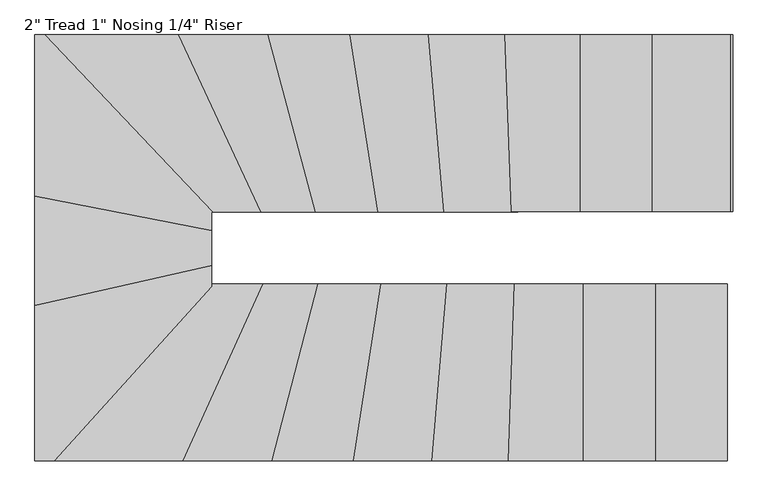
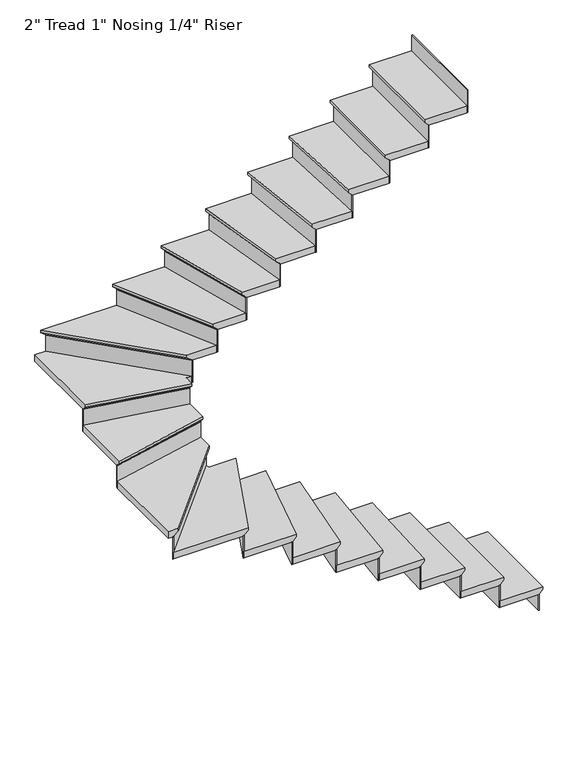
"""IFC4 building model written with IfcOpenShell, lengths in millimetres: stair flight geometry."""

from ifc_helpers import new_model, si_unit, origin, place, context, project, spatial, faceted_brep, source, transform, mapped, element, save


def stair_flight_7ceb0e75(model_context):
    return source(origin(), model_context, "Body", "Brep", [
        faceted_brep([(-10636.560337, -2913.3366944, 319.6166667), (-10636.560337, -2913.3366944, 338.6666667), (-10636.560337, -3599.1366944, 338.6666667), (-10636.560337, -3599.1366944, 319.6166667), (-10661.960337, -2913.3366944, 294.2166667), (-10661.960337, -3599.1366944, 294.2166667), (-10941.360337, -2913.3366944, 338.6666667), (-10941.360337, -3599.1366944, 338.6666667), (-10661.960337, -3599.1366944, 287.8666667), (-10941.360337, -3599.1366944, 287.8666667), (-10941.360337, -2913.3366944, 287.8666667), (-10661.960337, -2913.3366944, 287.8666667)], [[[0, 1, 2, 3]], [[4, 0, 3, 5]], [[2, 1, 6, 7]], [[8, 9, 10, 11]], [[2, 7, 9, 8, 5, 3]], [[8, 11, 4, 5]], [[6, 1, 0, 4, 11, 10]], [[7, 6, 10, 9]]]),
        faceted_brep([(-10661.960337, -2913.3366944, 287.8666667), (-10661.960337, -2913.3366944, 169.3333333), (-10668.310337, -2913.3366944, 169.3333333), (-10668.310337, -2913.3366944, 287.8666667), (-10661.960337, -3599.1366944, 287.8666667), (-10668.310337, -3599.1366944, 287.8666667), (-10668.310337, -3599.1366944, 169.3333333), (-10661.960337, -3599.1366944, 169.3333333)], [[[0, 1, 2, 3]], [[4, 5, 6, 7]], [[1, 0, 4, 7]], [[2, 1, 7, 6]], [[3, 2, 6, 5]], [[0, 3, 5, 4]]]),
        faceted_brep([(-10941.360337, -2913.3366944, 457.2), (-10941.360337, -2913.3366944, 287.8666667), (-10947.710337, -2913.3366944, 287.8666667), (-10947.710337, -2913.3366944, 457.2), (-10941.360337, -3599.1366944, 457.2), (-10947.710337, -3599.1366944, 457.2), (-10947.710337, -3599.1366944, 287.8666667), (-10941.360337, -3599.1366944, 287.8666667)], [[[0, 1, 2, 3]], [[4, 5, 6, 7]], [[1, 0, 4, 7]], [[2, 1, 7, 6]], [[3, 2, 6, 5]], [[0, 3, 5, 4]]]),
        faceted_brep([(-10915.960337, -3599.1366944, 508.0), (-10915.960337, -2913.3366944, 508.0), (-11220.760337, -2913.3366944, 508.0), (-11220.760337, -3599.1366944, 508.0), (-10941.360337, -3599.1366944, 457.2), (-11220.760337, -3599.1366944, 457.2), (-11220.760337, -2913.3366944, 457.2), (-10941.360337, -2913.3366944, 457.2), (-10941.360337, -3599.1366944, 463.55), (-10915.960337, -3599.1366944, 488.95), (-10941.360337, -2913.3366944, 463.55), (-10915.960337, -2913.3366944, 488.95)], [[[0, 1, 2, 3]], [[4, 5, 6, 7]], [[0, 3, 5, 4, 8, 9]], [[4, 7, 10, 8]], [[2, 1, 11, 10, 7, 6]], [[3, 2, 6, 5]], [[11, 1, 0, 9]], [[10, 11, 9, 8]]]),
        faceted_brep([(-11220.760337, -2913.3366944, 626.5333333), (-11220.760337, -2913.3366944, 457.2), (-11227.110337, -2913.3366944, 457.2), (-11227.110337, -2913.3366944, 626.5333333), (-11220.760337, -3599.1366944, 626.5333333), (-11227.110337, -3599.1366944, 626.5333333), (-11227.110337, -3599.1366944, 457.2), (-11220.760337, -3599.1366944, 457.2)], [[[0, 1, 2, 3]], [[4, 5, 6, 7]], [[1, 0, 4, 7]], [[2, 1, 7, 6]], [[3, 2, 6, 5]], [[0, 3, 5, 4]]]),
        faceted_brep([(-11195.360337, -3599.1366944, 677.3333333), (-11195.360337, -2913.3366944, 677.3333333), (-11487.9704957, -2913.3366944, 677.3333333), (-11512.3823522, -3599.1366944, 677.3333333), (-11220.760337, -3599.1366944, 626.5333333), (-11512.3823522, -3599.1366944, 626.5333333), (-11487.9704957, -2913.3366944, 626.5333333), (-11220.760337, -2913.3366944, 626.5333333), (-11220.760337, -3599.1366944, 632.8833333), (-11195.360337, -3599.1366944, 658.2833333), (-11220.760337, -2913.3366944, 632.8833333), (-11195.360337, -2913.3366944, 658.2833333)], [[[0, 1, 2, 3]], [[4, 5, 6, 7]], [[0, 3, 5, 4, 8, 9]], [[4, 7, 10, 8]], [[2, 1, 11, 10, 7, 6]], [[3, 2, 6, 5]], [[11, 1, 0, 9]], [[10, 11, 9, 8]]]),
        faceted_brep([(-11487.9704957, -2913.3366944, 795.8666667), (-11487.9704957, -2913.3366944, 626.5333333), (-11494.3245175, -2913.3366944, 626.5333333), (-11494.3245175, -2913.3366944, 795.8666667), (-11512.3823522, -3599.1366944, 795.8666667), (-11518.7363739, -3599.1366944, 795.8666667), (-11518.7363739, -3599.1366944, 626.5333333), (-11512.3823522, -3599.1366944, 626.5333333)], [[[0, 1, 2, 3]], [[4, 5, 6, 7]], [[1, 0, 4, 7]], [[2, 1, 7, 6]], [[3, 2, 6, 5]], [[0, 3, 5, 4]]]),
        faceted_brep([(-11486.9662653, -3599.1366944, 846.6666667), (-11462.5544088, -2913.3366944, 846.6666667), (-11750.8954257, -2913.3366944, 846.6666667), (-11808.403542, -3599.1366944, 846.6666667), (-11512.3823522, -3599.1366944, 795.8666667), (-11808.403542, -3599.1366944, 795.8666667), (-11750.8954257, -2913.3366944, 795.8666667), (-11487.9704957, -2913.3366944, 795.8666667), (-11512.3823522, -3599.1366944, 802.2166667), (-11486.9662653, -3599.1366944, 827.6166667), (-11487.9704957, -2913.3366944, 802.2166667), (-11462.5544088, -2913.3366944, 827.6166667)], [[[0, 1, 2, 3]], [[4, 5, 6, 7]], [[0, 3, 5, 4, 8, 9]], [[4, 7, 10, 8]], [[2, 1, 11, 10, 7, 6]], [[3, 2, 6, 5]], [[11, 1, 0, 9]], [[10, 11, 9, 8]]]),
        faceted_brep([(-11750.8954257, -2913.3366944, 965.2), (-11750.8954257, -2913.3366944, 795.8666667), (-11757.2677123, -2913.3366944, 795.8666667), (-11757.2677123, -2913.3366944, 965.2), (-11808.403542, -3599.1366944, 965.2), (-11814.7758287, -3599.1366944, 965.2), (-11814.7758287, -3599.1366944, 795.8666667), (-11808.403542, -3599.1366944, 795.8666667)], [[[0, 1, 2, 3]], [[4, 5, 6, 7]], [[1, 0, 4, 7]], [[2, 1, 7, 6]], [[3, 2, 6, 5]], [[0, 3, 5, 4]]]),
        faceted_brep([(-11782.9143952, -3599.1366944, 1016.0), (-11725.4062789, -2913.3366944, 1016.0), (-12006.7931198, -2913.3366944, 1016.0), (-12111.7186828, -3599.1366944, 1016.0), (-11808.403542, -3599.1366944, 965.2), (-12111.7186828, -3599.1366944, 965.2), (-12006.7931198, -2913.3366944, 965.2), (-11750.8954257, -2913.3366944, 965.2), (-11808.403542, -3599.1366944, 971.55), (-11782.9143952, -3599.1366944, 996.95), (-11750.8954257, -2913.3366944, 971.55), (-11725.4062789, -2913.3366944, 996.95)], [[[0, 1, 2, 3]], [[4, 5, 6, 7]], [[0, 3, 5, 4, 8, 9]], [[4, 7, 10, 8]], [[2, 1, 11, 10, 7, 6]], [[3, 2, 6, 5]], [[11, 1, 0, 9]], [[10, 11, 9, 8]]]),
        faceted_brep([(-12006.7931198, -2913.3366944, 1134.5333333), (-12006.7931198, -2913.3366944, 965.2), (-12013.2170109, -2913.3366944, 965.2), (-12013.2170109, -2913.3366944, 1134.5333333), (-12111.7186828, -3599.1366944, 1134.5333333), (-12118.1425738, -3599.1366944, 1134.5333333), (-12118.1425738, -3599.1366944, 965.2), (-12111.7186828, -3599.1366944, 965.2)], [[[0, 1, 2, 3]], [[4, 5, 6, 7]], [[1, 0, 4, 7]], [[2, 1, 7, 6]], [[3, 2, 6, 5]], [[0, 3, 5, 4]]]),
        faceted_brep([(-12086.0231185, -3599.1366944, 1185.3333333), (-11981.0975556, -2913.3366944, 1185.3333333), (-12249.9438364, -2913.3366944, 1185.3333333), (-12428.4698673, -3599.1366944, 1185.3333333), (-12111.7186828, -3599.1366944, 1134.5333333), (-12428.4698673, -3599.1366944, 1134.5333333), (-12249.9438364, -2913.3366944, 1134.5333333), (-12006.7931198, -2913.3366944, 1134.5333333), (-12111.7186828, -3599.1366944, 1140.8833333), (-12086.0231185, -3599.1366944, 1166.2833333), (-12006.7931198, -2913.3366944, 1140.8833333), (-11981.0975556, -2913.3366944, 1166.2833333)], [[[0, 1, 2, 3]], [[4, 5, 6, 7]], [[0, 3, 5, 4, 8, 9]], [[4, 7, 10, 8]], [[2, 1, 11, 10, 7, 6]], [[3, 2, 6, 5]], [[11, 1, 0, 9]], [[10, 11, 9, 8]]]),
        faceted_brep([(-12249.9438364, -2913.3366944, 1303.8666667), (-12249.9438364, -2913.3366944, 1134.5333333), (-12256.5054651, -2913.3366944, 1134.5333333), (-12256.5054651, -2913.3366944, 1303.8666667), (-12428.4698673, -3599.1366944, 1303.8666667), (-12435.031496, -3599.1366944, 1303.8666667), (-12435.031496, -3599.1366944, 1134.5333333), (-12428.4698673, -3599.1366944, 1134.5333333)], [[[0, 1, 2, 3]], [[4, 5, 6, 7]], [[1, 0, 4, 7]], [[2, 1, 7, 6]], [[3, 2, 6, 5]], [[0, 3, 5, 4]]]),
        faceted_brep([(-12402.2233525, -3599.1366944, 1354.6666667), (-12223.6973216, -2913.3366944, 1354.6666667), (-12466.0747967, -2913.3366944, 1354.6666667), (-12774.3420115, -3599.1366944, 1354.6666667), (-12428.4698673, -3599.1366944, 1303.8666667), (-12774.3420115, -3599.1366944, 1303.8666667), (-12466.0747967, -2913.3366944, 1303.8666667), (-12249.9438364, -2913.3366944, 1303.8666667), (-12428.4698673, -3599.1366944, 1310.2166667), (-12402.2233525, -3599.1366944, 1335.6166667), (-12249.9438364, -2913.3366944, 1310.2166667), (-12223.6973216, -2913.3366944, 1335.6166667)], [[[0, 1, 2, 3]], [[4, 5, 6, 7]], [[0, 3, 5, 4, 8, 9]], [[4, 7, 10, 8]], [[2, 1, 11, 10, 7, 6]], [[3, 2, 6, 5]], [[11, 1, 0, 9]], [[10, 11, 9, 8]]]),
        faceted_brep([(-12466.0747967, -2913.3366944, 1473.2), (-12466.0747967, -2913.3366944, 1303.8666667), (-12473.0368134, -2913.3366944, 1303.8666667), (-12473.0368134, -2913.3366944, 1473.2), (-12774.3420115, -3599.1366944, 1473.2), (-12781.3040282, -3599.1366944, 1473.2), (-12781.3040282, -3599.1366944, 1303.8666667), (-12774.3420115, -3599.1366944, 1303.8666667)], [[[0, 1, 2, 3]], [[4, 5, 6, 7]], [[1, 0, 4, 7]], [[2, 1, 7, 6]], [[3, 2, 6, 5]], [[0, 3, 5, 4]]]),
        faceted_brep([(-12746.4939444, -3599.1366944, 1524.0), (-12438.2267296, -2913.3366944, 1524.0), (-12633.931213, -2913.3366944, 1524.0), (-12633.931213, -2885.7746547, 1524.0), (-13279.3628435, -3599.1366944, 1524.0), (-12774.3420115, -3599.1366944, 1473.2), (-13279.3628435, -3599.1366944, 1473.2), (-12633.931213, -2885.7746547, 1473.2), (-12633.931213, -2913.3366944, 1473.2), (-12466.0747967, -2913.3366944, 1473.2), (-12774.3420115, -3599.1366944, 1479.55), (-12746.4939444, -3599.1366944, 1504.95), (-12466.0747967, -2913.3366944, 1479.55), (-12438.2267296, -2913.3366944, 1504.95)], [[[0, 1, 2, 3, 4]], [[5, 6, 7, 8, 9]], [[0, 4, 6, 5, 10, 11]], [[5, 9, 12, 10]], [[3, 2, 8, 7]], [[4, 3, 7, 6]], [[13, 1, 0, 11]], [[12, 13, 11, 10]], [[2, 1, 13, 12, 9, 8]]]),
        faceted_brep([(-12633.931213, -2885.7746547, 1642.5333333), (-12633.931213, -2885.7746547, 1473.2), (-12633.931213, -2876.310016, 1473.2), (-12633.931213, -2876.310016, 1642.5333333), (-13279.3628435, -3599.1366944, 1642.5333333), (-13287.9262052, -3599.1366944, 1642.5333333), (-13287.9262052, -3599.1366944, 1473.2), (-13279.3628435, -3599.1366944, 1473.2)], [[[0, 1, 2, 3]], [[4, 5, 6, 7]], [[1, 0, 4, 7]], [[2, 1, 7, 6]], [[3, 2, 6, 5]], [[0, 3, 5, 4]]]),
        faceted_brep([(-13319.731213, -2969.8773999, 1693.3333333), (-13319.731213, -3599.1366944, 1693.3333333), (-13245.1093966, -3599.1366944, 1693.3333333), (-12633.931213, -2923.6332096, 1693.3333333), (-12633.931213, -2815.9096738, 1693.3333333), (-13319.731213, -3599.1366944, 1642.5333333), (-13319.731213, -2969.8773999, 1642.5333333), (-12633.931213, -2815.9096738, 1642.5333333), (-12633.931213, -2885.7746547, 1642.5333333), (-13279.3628435, -3599.1366944, 1642.5333333), (-12633.931213, -2885.7746547, 1648.8833333), (-13279.3628435, -3599.1366944, 1648.8833333), (-12633.931213, -2923.6332096, 1674.2833333), (-13245.1093966, -3599.1366944, 1674.2833333)], [[[0, 1, 2, 3, 4]], [[5, 6, 7, 8, 9]], [[1, 0, 6, 5]], [[9, 8, 10, 11]], [[0, 4, 7, 6]], [[12, 3, 2, 13]], [[10, 12, 13, 11]], [[2, 1, 5, 9, 11, 13]], [[4, 3, 12, 10, 8, 7]]]),
        faceted_brep([(-12633.931213, -2815.9096738, 1811.8666667), (-12633.931213, -2815.9096738, 1642.5333333), (-12633.931213, -2809.4016086, 1642.5333333), (-12633.931213, -2809.4016086, 1811.8666667), (-13319.731213, -2969.8773999, 1811.8666667), (-13319.731213, -2963.3693347, 1811.8666667), (-13319.731213, -2963.3693347, 1642.5333333), (-13319.731213, -2969.8773999, 1642.5333333)], [[[0, 1, 2, 3]], [[4, 5, 6, 7]], [[1, 0, 4, 7]], [[2, 1, 7, 6]], [[3, 2, 6, 5]], [[0, 3, 5, 4]]]),
        faceted_brep([(-13319.731213, -2995.9096606, 1862.6666667), (-12633.931213, -2841.9419345, 1862.6666667), (-12633.931213, -2679.8898045, 1862.6666667), (-13319.731213, -2547.4021429, 1862.6666667), (-13319.731213, -2969.8773999, 1811.8666667), (-13319.731213, -2547.4021429, 1811.8666667), (-12633.931213, -2679.8898045, 1811.8666667), (-12633.931213, -2815.9096738, 1811.8666667), (-13319.731213, -2969.8773999, 1818.2166667), (-13319.731213, -2995.9096606, 1843.6166667), (-12633.931213, -2815.9096738, 1818.2166667), (-12633.931213, -2841.9419345, 1843.6166667)], [[[0, 1, 2, 3]], [[4, 5, 6, 7]], [[0, 3, 5, 4, 8, 9]], [[4, 7, 10, 8]], [[2, 1, 11, 10, 7, 6]], [[3, 2, 6, 5]], [[11, 1, 0, 9]], [[10, 11, 9, 8]]]),
        faceted_brep([(-12633.931213, -2679.8898045, 1981.2), (-12633.931213, -2679.8898045, 1811.8666667), (-12633.931213, -2673.4223951, 1811.8666667), (-12633.931213, -2673.4223951, 1981.2), (-13319.731213, -2547.4021429, 1981.2), (-13319.731213, -2540.9347334, 1981.2), (-13319.731213, -2540.9347334, 1811.8666667), (-13319.731213, -2547.4021429, 1811.8666667)], [[[0, 1, 2, 3]], [[4, 5, 6, 7]], [[1, 0, 4, 7]], [[2, 1, 7, 6]], [[3, 2, 6, 5]], [[0, 3, 5, 4]]]),
        faceted_brep([(-13243.8610988, -1948.1366944, 2032.0), (-13319.731213, -1948.1366944, 2032.0), (-13319.731213, -2573.2717807, 2032.0), (-12633.931213, -2705.7594424, 2032.0), (-12633.931213, -2633.9366944, 2032.0), (-12593.8868071, -2633.9366944, 2032.0), (-13319.731213, -1948.1366944, 1981.2), (-13243.8610988, -1948.1366944, 1981.2), (-12593.8868071, -2633.9366944, 1981.2), (-12633.931213, -2633.9366944, 1981.2), (-12633.931213, -2679.8898045, 1981.2), (-13319.731213, -2547.4021429, 1981.2), (-13319.731213, -2547.4021429, 1987.55), (-13319.731213, -2573.2717807, 2012.95), (-12633.931213, -2679.8898045, 1987.55), (-12633.931213, -2705.7594424, 2012.95)], [[[0, 1, 2, 3, 4, 5]], [[6, 7, 8, 9, 10, 11]], [[1, 0, 7, 6]], [[2, 1, 6, 11, 12, 13]], [[11, 10, 14, 12]], [[4, 3, 15, 14, 10, 9]], [[0, 5, 8, 7]], [[15, 3, 2, 13]], [[14, 15, 13, 12]], [[5, 4, 9, 8]]]),
        faceted_brep([(-12593.8868071, -2633.9366944, 2150.5333333), (-12593.8868071, -2633.9366944, 1981.2), (-12585.1379672, -2633.9366944, 1981.2), (-12585.1379672, -2633.9366944, 2150.5333333), (-13243.8610988, -1948.1366944, 2150.5333333), (-13235.1122589, -1948.1366944, 2150.5333333), (-13235.1122589, -1948.1366944, 1981.2), (-13243.8610988, -1948.1366944, 1981.2)], [[[0, 1, 2, 3]], [[4, 5, 6, 7]], [[1, 0, 4, 7]], [[2, 1, 7, 6]], [[3, 2, 6, 5]], [[0, 3, 5, 4]]]),
        faceted_brep([(-13278.8564585, -1948.1366944, 2201.3333333), (-12628.8821668, -2633.9366944, 2201.3333333), (-12415.318386, -2633.9366944, 2201.3333333), (-12734.933264, -1948.1366944, 2201.3333333), (-13243.8610988, -1948.1366944, 2150.5333333), (-12734.933264, -1948.1366944, 2150.5333333), (-12415.318386, -2633.9366944, 2150.5333333), (-12593.8868071, -2633.9366944, 2150.5333333), (-13243.8610988, -1948.1366944, 2156.8833333), (-13278.8564585, -1948.1366944, 2182.2833333), (-12593.8868071, -2633.9366944, 2156.8833333), (-12628.8821668, -2633.9366944, 2182.2833333)], [[[0, 1, 2, 3]], [[4, 5, 6, 7]], [[0, 3, 5, 4, 8, 9]], [[4, 7, 10, 8]], [[2, 1, 11, 10, 7, 6]], [[3, 2, 6, 5]], [[11, 1, 0, 9]], [[10, 11, 9, 8]]]),
        faceted_brep([(-12415.318386, -2633.9366944, 2319.8666667), (-12415.318386, -2633.9366944, 2150.5333333), (-12408.3126362, -2633.9366944, 2150.5333333), (-12408.3126362, -2633.9366944, 2319.8666667), (-12734.933264, -1948.1366944, 2319.8666667), (-12727.9275142, -1948.1366944, 2319.8666667), (-12727.9275142, -1948.1366944, 2150.5333333), (-12734.933264, -1948.1366944, 2150.5333333)], [[[0, 1, 2, 3]], [[4, 5, 6, 7]], [[1, 0, 4, 7]], [[2, 1, 7, 6]], [[3, 2, 6, 5]], [[0, 3, 5, 4]]]),
        faceted_brep([(-12762.9562633, -1948.1366944, 2370.6666667), (-12443.3413854, -2633.9366944, 2370.6666667), (-12205.1244137, -2633.9366944, 2370.6666667), (-12389.76429, -1948.1366944, 2370.6666667), (-12734.933264, -1948.1366944, 2319.8666667), (-12389.76429, -1948.1366944, 2319.8666667), (-12205.1244137, -2633.9366944, 2319.8666667), (-12415.318386, -2633.9366944, 2319.8666667), (-12734.933264, -1948.1366944, 2326.2166667), (-12762.9562633, -1948.1366944, 2351.6166667), (-12415.318386, -2633.9366944, 2326.2166667), (-12443.3413854, -2633.9366944, 2351.6166667)], [[[0, 1, 2, 3]], [[4, 5, 6, 7]], [[0, 3, 5, 4, 8, 9]], [[4, 7, 10, 8]], [[2, 1, 11, 10, 7, 6]], [[3, 2, 6, 5]], [[11, 1, 0, 9]], [[10, 11, 9, 8]]]),
        faceted_brep([(-12205.1244137, -2633.9366944, 2489.2), (-12205.1244137, -2633.9366944, 2319.8666667), (-12198.5482956, -2633.9366944, 2319.8666667), (-12198.5482956, -2633.9366944, 2489.2), (-12389.76429, -1948.1366944, 2489.2), (-12383.1881719, -1948.1366944, 2489.2), (-12383.1881719, -1948.1366944, 2319.8666667), (-12389.76429, -1948.1366944, 2319.8666667)], [[[0, 1, 2, 3]], [[4, 5, 6, 7]], [[1, 0, 4, 7]], [[2, 1, 7, 6]], [[3, 2, 6, 5]], [[0, 3, 5, 4]]]),
        faceted_brep([(-12416.0687625, -1948.1366944, 2540.0), (-12231.4288862, -2633.9366944, 2540.0), (-11964.4502805, -2633.9366944, 2540.0), (-12072.8170712, -1948.1366944, 2540.0), (-12389.76429, -1948.1366944, 2489.2), (-12072.8170712, -1948.1366944, 2489.2), (-11964.4502805, -2633.9366944, 2489.2), (-12205.1244137, -2633.9366944, 2489.2), (-12389.76429, -1948.1366944, 2495.55), (-12416.0687625, -1948.1366944, 2520.95), (-12205.1244137, -2633.9366944, 2495.55), (-12231.4288862, -2633.9366944, 2520.95)], [[[0, 1, 2, 3]], [[4, 5, 6, 7]], [[0, 3, 5, 4, 8, 9]], [[4, 7, 10, 8]], [[2, 1, 11, 10, 7, 6]], [[3, 2, 6, 5]], [[11, 1, 0, 9]], [[10, 11, 9, 8]]]),
        faceted_brep([(-11964.4502805, -2633.9366944, 2658.5333333), (-11964.4502805, -2633.9366944, 2489.2), (-11958.0214934, -2633.9366944, 2489.2), (-11958.0214934, -2633.9366944, 2658.5333333), (-12072.8170712, -1948.1366944, 2658.5333333), (-12066.388284, -1948.1366944, 2658.5333333), (-12066.388284, -1948.1366944, 2489.2), (-12072.8170712, -1948.1366944, 2489.2)], [[[0, 1, 2, 3]], [[4, 5, 6, 7]], [[1, 0, 4, 7]], [[2, 1, 7, 6]], [[3, 2, 6, 5]], [[0, 3, 5, 4]]]),
        faceted_brep([(-12098.5322197, -1948.1366944, 2709.3333333), (-11990.165429, -2633.9366944, 2709.3333333), (-11709.7836039, -2633.9366944, 2709.3333333), (-11769.124229, -1948.1366944, 2709.3333333), (-12072.8170712, -1948.1366944, 2658.5333333), (-11769.124229, -1948.1366944, 2658.5333333), (-11709.7836039, -2633.9366944, 2658.5333333), (-11964.4502805, -2633.9366944, 2658.5333333), (-12072.8170712, -1948.1366944, 2664.8833333), (-12098.5322197, -1948.1366944, 2690.2833333), (-11964.4502805, -2633.9366944, 2664.8833333), (-11990.165429, -2633.9366944, 2690.2833333)], [[[0, 1, 2, 3]], [[4, 5, 6, 7]], [[0, 3, 5, 4, 8, 9]], [[4, 7, 10, 8]], [[2, 1, 11, 10, 7, 6]], [[3, 2, 6, 5]], [[11, 1, 0, 9]], [[10, 11, 9, 8]]]),
        faceted_brep([(-11709.7836039, -2633.9366944, 2827.8666667), (-11709.7836039, -2633.9366944, 2658.5333333), (-11703.4098769, -2633.9366944, 2658.5333333), (-11703.4098769, -2633.9366944, 2827.8666667), (-11769.124229, -1948.1366944, 2827.8666667), (-11762.750502, -1948.1366944, 2827.8666667), (-11762.750502, -1948.1366944, 2658.5333333), (-11769.124229, -1948.1366944, 2658.5333333)], [[[0, 1, 2, 3]], [[4, 5, 6, 7]], [[1, 0, 4, 7]], [[2, 1, 7, 6]], [[3, 2, 6, 5]], [[0, 3, 5, 4]]]),
        faceted_brep([(-11794.6191369, -1948.1366944, 2878.6666667), (-11735.2785118, -2633.9366944, 2878.6666667), (-11447.5447698, -2633.9366944, 2878.6666667), (-11472.7186658, -1948.1366944, 2878.6666667), (-11769.124229, -1948.1366944, 2827.8666667), (-11472.7186658, -1948.1366944, 2827.8666667), (-11447.5447698, -2633.9366944, 2827.8666667), (-11709.7836039, -2633.9366944, 2827.8666667), (-11769.124229, -1948.1366944, 2834.2166667), (-11794.6191369, -1948.1366944, 2859.6166667), (-11709.7836039, -2633.9366944, 2834.2166667), (-11735.2785118, -2633.9366944, 2859.6166667)], [[[0, 1, 2, 3]], [[4, 5, 6, 7]], [[0, 3, 5, 4, 8, 9]], [[4, 7, 10, 8]], [[2, 1, 11, 10, 7, 6]], [[3, 2, 6, 5]], [[11, 1, 0, 9]], [[10, 11, 9, 8]]]),
        faceted_brep([(-11447.5447698, -2633.9366944, 2997.2), (-11447.5447698, -2633.9366944, 2827.8666667), (-11441.1904931, -2633.9366944, 2827.8666667), (-11441.1904931, -2633.9366944, 2997.2), (-11472.7186658, -1948.1366944, 2997.2), (-11466.3643891, -1948.1366944, 2997.2), (-11466.3643891, -1948.1366944, 2827.8666667), (-11472.7186658, -1948.1366944, 2827.8666667)], [[[0, 1, 2, 3]], [[4, 5, 6, 7]], [[1, 0, 4, 7]], [[2, 1, 7, 6]], [[3, 2, 6, 5]], [[0, 3, 5, 4]]]),
        faceted_brep([(-11498.1357723, -1948.1366944, 3048.0), (-11472.9618764, -2633.9366944, 3048.0), (-11180.7488243, -2633.9366944, 3048.0), (-11180.7488243, -1948.1366944, 3048.0), (-11472.7186658, -1948.1366944, 2997.2), (-11180.7488243, -1948.1366944, 2997.2), (-11180.7488243, -2633.9366944, 2997.2), (-11447.5447698, -2633.9366944, 2997.2), (-11472.7186658, -1948.1366944, 3003.55), (-11498.1357723, -1948.1366944, 3028.95), (-11447.5447698, -2633.9366944, 3003.55), (-11472.9618764, -2633.9366944, 3028.95)], [[[0, 1, 2, 3]], [[4, 5, 6, 7]], [[0, 3, 5, 4, 8, 9]], [[4, 7, 10, 8]], [[2, 1, 11, 10, 7, 6]], [[3, 2, 6, 5]], [[11, 1, 0, 9]], [[10, 11, 9, 8]]]),
        faceted_brep([(-11180.7488243, -2633.9366944, 3166.5333333), (-11180.7488243, -2633.9366944, 2997.2), (-11174.3988243, -2633.9366944, 2997.2), (-11174.3988243, -2633.9366944, 3166.5333333), (-11180.7488243, -1948.1366944, 3166.5333333), (-11174.3988243, -1948.1366944, 3166.5333333), (-11174.3988243, -1948.1366944, 2997.2), (-11180.7488243, -1948.1366944, 2997.2)], [[[0, 1, 2, 3]], [[4, 5, 6, 7]], [[1, 0, 4, 7]], [[2, 1, 7, 6]], [[3, 2, 6, 5]], [[0, 3, 5, 4]]]),
        faceted_brep([(-11206.1488243, -1948.1366944, 3217.3333333), (-11206.1488243, -2633.9366944, 3217.3333333), (-10901.3488243, -2633.9366944, 3217.3333333), (-10901.3488243, -1948.1366944, 3217.3333333), (-11180.7488243, -1948.1366944, 3166.5333333), (-10901.3488243, -1948.1366944, 3166.5333333), (-10901.3488243, -2633.9366944, 3166.5333333), (-11180.7488243, -2633.9366944, 3166.5333333), (-11180.7488243, -1948.1366944, 3172.8833333), (-11206.1488243, -1948.1366944, 3198.2833333), (-11180.7488243, -2633.9366944, 3172.8833333), (-11206.1488243, -2633.9366944, 3198.2833333)], [[[0, 1, 2, 3]], [[4, 5, 6, 7]], [[0, 3, 5, 4, 8, 9]], [[4, 7, 10, 8]], [[2, 1, 11, 10, 7, 6]], [[3, 2, 6, 5]], [[11, 1, 0, 9]], [[10, 11, 9, 8]]]),
        faceted_brep([(-10901.3488243, -2633.9366944, 3335.8666667), (-10901.3488243, -2633.9366944, 3166.5333333), (-10894.9988243, -2633.9366944, 3166.5333333), (-10894.9988243, -2633.9366944, 3335.8666667), (-10901.3488243, -1948.1366944, 3335.8666667), (-10894.9988243, -1948.1366944, 3335.8666667), (-10894.9988243, -1948.1366944, 3166.5333333), (-10901.3488243, -1948.1366944, 3166.5333333)], [[[0, 1, 2, 3]], [[4, 5, 6, 7]], [[1, 0, 4, 7]], [[2, 1, 7, 6]], [[3, 2, 6, 5]], [[0, 3, 5, 4]]]),
        faceted_brep([(-10621.9488243, -2633.9366944, 3505.2), (-10621.9488243, -2633.9366944, 3335.8666667), (-10615.5988243, -2633.9366944, 3335.8666667), (-10615.5988243, -2633.9366944, 3505.2), (-10621.9488243, -1948.1366944, 3505.2), (-10615.5988243, -1948.1366944, 3505.2), (-10615.5988243, -1948.1366944, 3335.8666667), (-10621.9488243, -1948.1366944, 3335.8666667)], [[[0, 1, 2, 3]], [[4, 5, 6, 7]], [[1, 0, 4, 7]], [[2, 1, 7, 6]], [[3, 2, 6, 5]], [[0, 3, 5, 4]]]),
        faceted_brep([(-10926.7488243, -1948.1366944, 3386.6666667), (-10926.7488243, -2633.9366944, 3386.6666667), (-10621.9488243, -2633.9366944, 3386.6666667), (-10621.9488243, -1948.1366944, 3386.6666667), (-10901.3488243, -1948.1366944, 3335.8666667), (-10621.9488243, -1948.1366944, 3335.8666667), (-10621.9488243, -2633.9366944, 3335.8666667), (-10901.3488243, -2633.9366944, 3335.8666667), (-10901.3488243, -1948.1366944, 3342.2166667), (-10926.7488243, -1948.1366944, 3367.6166667), (-10901.3488243, -2633.9366944, 3342.2166667), (-10926.7488243, -2633.9366944, 3367.6166667)], [[[0, 1, 2, 3]], [[4, 5, 6, 7]], [[0, 3, 5, 4, 8, 9]], [[4, 7, 10, 8]], [[2, 1, 11, 10, 7, 6]], [[3, 2, 6, 5]], [[11, 1, 0, 9]], [[10, 11, 9, 8]]]),
    ])


if __name__ == "__main__":
    model = new_model("IFC4")
    model_context = context("Model", 3, world=origin())
    ifc_project = project(units=[si_unit("LENGTHUNIT", "METRE", prefix="MILLI")], contexts=[model_context])
    site = spatial("IfcSite", under=ifc_project)
    building = spatial("IfcBuilding", under=site)
    placement = place(None, origin())
    stair_flight_shape = stair_flight_7ceb0e75(model_context)
    element("IfcStairFlight", 1, ObjectType="2\" Tread 1\" Nosing 1/4\" Riser", at=placement, inside=building, context=model_context, shape_type="MappedRepresentation", body=[
        mapped(stair_flight_shape, transform((0.0, 0.0, 0.0), x_axis=(1.0, 0.0, 0.0), y_axis=(0.0, 1.0, 0.0), z_axis=(0.0, 0.0, 1.0))),
    ])
    save(model, "model.ifc")
